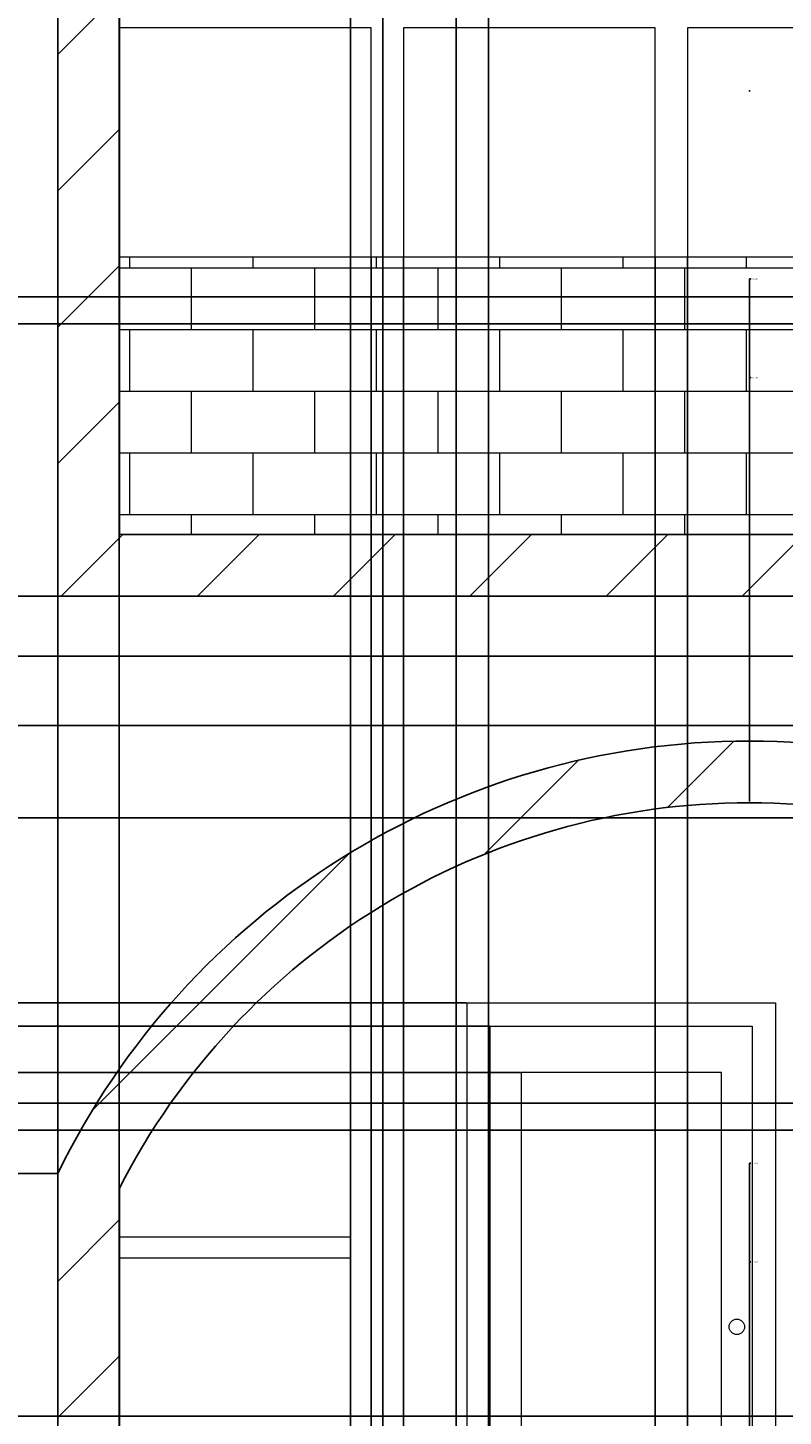
# Model space of a CAD drawing. Units: inches. Extents: x -14 to 375, y -86 to 549.
# Tile 7 of 12: x 130 to 228, y 156 to 336. Entities that reach past the tile are written whole.
import ezdxf

# ---------------------------------------------------------------- set-up
doc = ezdxf.new("R2010")
doc.units = ezdxf.units.IN
doc.header["$MEASUREMENT"] = 0
for name, color, linetype, lineweight in [('A-ANNO-DIMS', 2, 'Continuous', 18), ('A-DOOR', 3, 'Continuous', 18), ('A-ELEV', 7, 'Continuous', 25), ('A-ELEV-PATT', 8, 'Continuous', 13), ('A-ELEV-RAIL', 8, 'Continuous', 18), ('A-GLAZ', 4, 'Continuous', 18)]:
    doc.layers.add(name, color=color, linetype=linetype, lineweight=lineweight)
doc.styles.get("Standard").update_dxf_attribs({"font": 'arial.ttf'})
doc.dimstyles.get("Standard").update_dxf_attribs({"dimtxt": 0.18, "dimasz": 0.18, "dimexe": 0.18, "dimexo": 0.0625, "dimgap": 0.09, "dimtad": 0, "dimtih": 1, "dimtoh": 1, "dimdec": 4, "dimzin": 0, "dimdsep": 46, "dimtxsty": 'Standard', "dimcen": 0.09, "dimadec": 0, "dimazin": 0, "dimtfac": 1, "dimtdec": 4, "dimtofl": 0, "dimtmove": 0, "dimatfit": 3, "dimfxl": 1, "dimtolj": 1, "dimtzin": 0, "dimarcsym": 0})

# ---------------------------------------------------------------- blocks, each defined once
blk = doc.blocks.new('*U3')
blk.add_lwpolyline([(3.12, 0.01), (0.12, 0.01), (0.12, 84.01), (40.12, 84.01), (40.12, 0.01), (37.12, 0.01)])
for points in [[(37.12, 80.99), (37.12, 0.01), (3.12, 0.01), (3.12, 80.99)], [(33.12, 6.01), (33.12, 74.99), (7.12, 74.99), (7.12, 6.01)]]:
    blk.add_lwpolyline(points, close=True)
blk.add_circle((35.12, 42.01), 1)
blk = doc.blocks.new('*D15')
at = {"layer": 'A-ANNO-DIMS', "color": 0, "lineweight": -2, "transparency": 16777216}
for p, q in [((134.17, 187.85), (-13.88, 187.85)), ((-13.7, 187.67), (-13.7, 170.29)), ((-13.7, 152.56), (-13.7, 169.93)), ((38.44, 152.38), (-13.88, 152.38))]:
    blk.add_line(p, q, dxfattribs=at)
at = {"layer": 'A-ANNO-DIMS', "color": 0, "transparency": 16777216}
for points in [[(-13.73, 187.67), (-13.67, 187.67), (-13.7, 187.85)], [(-13.73, 152.56), (-13.67, 152.56), (-13.7, 152.38)]]:
    blk.add_solid(points, dxfattribs=at)
at = {"layer": 'Defpoints', "color": 0, "transparency": 16777216}
for p in [(-13.7, 187.85), (134.23, 187.85), (38.5, 152.38)]:
    blk.add_point(p, dxfattribs=at)
at = {"layer": 'A-ANNO-DIMS', "color": 0, "transparency": 16777216, "insert": (-13.7, 170.11), "char_height": 0.18, "attachment_point": 5}
blk.add_mtext('\\A1;35.47', dxfattribs=at)
blk = doc.blocks.new('*D16')
at = {"layer": 'A-ANNO-DIMS', "color": 0, "lineweight": -2, "transparency": 16777216}
for p, q in [((134.17, 262.71), (-13.88, 262.71)), ((-13.7, 262.53), (-13.7, 225.46)), ((-13.7, 188.03), (-13.7, 225.09)), ((134.17, 187.85), (-13.88, 187.85))]:
    blk.add_line(p, q, dxfattribs=at)
at = {"layer": 'A-ANNO-DIMS', "color": 0, "transparency": 16777216}
for points in [[(-13.73, 262.53), (-13.67, 262.53), (-13.7, 262.71)], [(-13.73, 188.03), (-13.67, 188.03), (-13.7, 187.85)]]:
    blk.add_solid(points, dxfattribs=at)
at = {"layer": 'Defpoints', "color": 0, "transparency": 16777216}
for p in [(-13.7, 262.71), (134.23, 262.71), (134.23, 187.85)]:
    blk.add_point(p, dxfattribs=at)
at = {"layer": 'A-ANNO-DIMS', "color": 0, "transparency": 16777216, "insert": (-13.7, 225.28), "char_height": 0.18, "attachment_point": 5}
blk.add_mtext('\\A1;74.86', dxfattribs=at)
blk = doc.blocks.new('*D17')
at = {"layer": 'A-ANNO-DIMS', "color": 0, "lineweight": -2, "transparency": 16777216}
for p, q in [((38.44, 432.97), (-13.88, 432.97)), ((-13.7, 432.79), (-13.7, 348.02)), ((-13.7, 262.89), (-13.7, 347.66)), ((134.17, 262.71), (-13.88, 262.71))]:
    blk.add_line(p, q, dxfattribs=at)
at = {"layer": 'A-ANNO-DIMS', "color": 0, "transparency": 16777216}
for points in [[(-13.73, 432.79), (-13.67, 432.79), (-13.7, 432.97)], [(-13.73, 262.89), (-13.67, 262.89), (-13.7, 262.71)]]:
    blk.add_solid(points, dxfattribs=at)
at = {"layer": 'Defpoints', "color": 0, "transparency": 16777216}
for p in [(-13.7, 432.97), (38.5, 432.97), (134.23, 262.71)]:
    blk.add_point(p, dxfattribs=at)
at = {"layer": 'A-ANNO-DIMS', "color": 0, "transparency": 16777216, "insert": (-13.7, 347.84), "char_height": 0.18, "attachment_point": 5}
blk.add_mtext('\\A1;170.26', dxfattribs=at)
blk = doc.blocks.new('*D29')
at = {"layer": 'A-ANNO-DIMS', "color": 0, "lineweight": -2, "transparency": 16777216}
for p, q in [((107.74, 193.48), (374.54, 193.48)), ((374.36, 193.3), (374.36, 175.11)), ((374.36, 156.56), (374.36, 174.75)), ((107.76, 156.38), (374.54, 156.38))]:
    blk.add_line(p, q, dxfattribs=at)
at = {"layer": 'A-ANNO-DIMS', "color": 0, "transparency": 16777216}
for points in [[(374.33, 193.3), (374.39, 193.3), (374.36, 193.48)], [(374.33, 156.56), (374.39, 156.56), (374.36, 156.38)]]:
    blk.add_solid(points, dxfattribs=at)
at = {"layer": 'Defpoints', "color": 0, "transparency": 16777216}
for p in [(107.68, 193.48), (374.36, 193.48), (107.7, 156.38)]:
    blk.add_point(p, dxfattribs=at)
at = {"layer": 'A-ANNO-DIMS', "color": 0, "transparency": 16777216, "insert": (374.36, 174.93), "char_height": 0.18, "attachment_point": 5}
blk.add_mtext('\\A1;37.106', dxfattribs=at)
blk = doc.blocks.new('*D30')
at = {"layer": 'A-ANNO-DIMS', "color": 0, "lineweight": -2, "transparency": 16777216}
for p, q in [((107.74, 196.98), (374.54, 196.98)), ((374.36, 196.8), (374.36, 195.41)), ((374.36, 193.66), (374.36, 195.05)), ((107.74, 193.48), (374.54, 193.48))]:
    blk.add_line(p, q, dxfattribs=at)
at = {"layer": 'A-ANNO-DIMS', "color": 0, "transparency": 16777216}
for points in [[(374.33, 196.8), (374.39, 196.8), (374.36, 196.98)], [(374.33, 193.66), (374.39, 193.66), (374.36, 193.48)]]:
    blk.add_solid(points, dxfattribs=at)
at = {"layer": 'Defpoints', "color": 0, "transparency": 16777216}
for p in [(107.68, 196.98), (374.36, 196.98), (107.68, 193.48)]:
    blk.add_point(p, dxfattribs=at)
at = {"layer": 'A-ANNO-DIMS', "color": 0, "transparency": 16777216, "insert": (374.36, 195.23), "char_height": 0.18, "attachment_point": 5}
blk.add_mtext('\\A1;3.501', dxfattribs=at)
blk = doc.blocks.new('*D31')
at = {"layer": 'A-ANNO-DIMS', "color": 0, "lineweight": -2, "transparency": 16777216}
for p, q in [((107.76, 233.96), (374.54, 233.96)), ((374.36, 233.78), (374.36, 215.65)), ((374.36, 197.16), (374.36, 215.29)), ((107.74, 196.98), (374.54, 196.98))]:
    blk.add_line(p, q, dxfattribs=at)
at = {"layer": 'A-ANNO-DIMS', "color": 0, "transparency": 16777216}
for points in [[(374.33, 233.78), (374.39, 233.78), (374.36, 233.96)], [(374.33, 197.16), (374.39, 197.16), (374.36, 196.98)]]:
    blk.add_solid(points, dxfattribs=at)
at = {"layer": 'Defpoints', "color": 0, "transparency": 16777216}
for p in [(107.7, 233.96), (374.36, 233.96), (107.68, 196.98)]:
    blk.add_point(p, dxfattribs=at)
at = {"layer": 'A-ANNO-DIMS', "color": 0, "transparency": 16777216, "insert": (374.36, 215.47), "char_height": 0.18, "attachment_point": 5}
blk.add_mtext('\\A1;36.975', dxfattribs=at)
blk = doc.blocks.new('*D32')
at = {"layer": 'A-ANNO-DIMS', "color": 0, "lineweight": -2, "transparency": 16777216}
for p, q in [((107.76, 245.96), (374.54, 245.96)), ((374.36, 245.78), (374.36, 240.14)), ((374.36, 234.14), (374.36, 239.78)), ((107.76, 233.96), (374.54, 233.96))]:
    blk.add_line(p, q, dxfattribs=at)
at = {"layer": 'A-ANNO-DIMS', "color": 0, "transparency": 16777216}
for points in [[(374.33, 245.78), (374.39, 245.78), (374.36, 245.96)], [(374.33, 234.14), (374.39, 234.14), (374.36, 233.96)]]:
    blk.add_solid(points, dxfattribs=at)
at = {"layer": 'Defpoints', "color": 0, "transparency": 16777216}
for p in [(107.7, 245.96), (374.36, 245.96), (107.7, 233.96)]:
    blk.add_point(p, dxfattribs=at)
at = {"layer": 'A-ANNO-DIMS', "color": 0, "transparency": 16777216, "insert": (374.36, 239.96), "char_height": 0.18, "attachment_point": 5}
blk.add_mtext('\\A1;12', dxfattribs=at)
blk = doc.blocks.new('*D33')
at = {"layer": 'A-ANNO-DIMS', "color": 0, "lineweight": -2, "transparency": 16777216}
for p, q in [((107.76, 254.96), (374.54, 254.96)), ((374.36, 254.78), (374.36, 250.64)), ((374.36, 246.14), (374.36, 250.28)), ((107.76, 245.96), (374.54, 245.96))]:
    blk.add_line(p, q, dxfattribs=at)
at = {"layer": 'A-ANNO-DIMS', "color": 0, "transparency": 16777216}
for points in [[(374.33, 254.78), (374.39, 254.78), (374.36, 254.96)], [(374.33, 246.14), (374.39, 246.14), (374.36, 245.96)]]:
    blk.add_solid(points, dxfattribs=at)
at = {"layer": 'Defpoints', "color": 0, "transparency": 16777216}
for p in [(107.7, 254.96), (374.36, 254.96), (107.7, 245.96)]:
    blk.add_point(p, dxfattribs=at)
at = {"layer": 'A-ANNO-DIMS', "color": 0, "transparency": 16777216, "insert": (374.36, 250.46), "char_height": 0.18, "attachment_point": 5}
blk.add_mtext('\\A1;9', dxfattribs=at)
blk = doc.blocks.new('*D34')
at = {"layer": 'A-ANNO-DIMS', "color": 0, "lineweight": -2, "transparency": 16777216}
for p, q in [((107.64, 298.04), (374.54, 298.04)), ((374.36, 297.86), (374.36, 276.68)), ((374.36, 255.14), (374.36, 276.32)), ((107.76, 254.96), (374.54, 254.96))]:
    blk.add_line(p, q, dxfattribs=at)
at = {"layer": 'A-ANNO-DIMS', "color": 0, "transparency": 16777216}
for points in [[(374.33, 297.86), (374.39, 297.86), (374.36, 298.04)], [(374.33, 255.14), (374.39, 255.14), (374.36, 254.96)]]:
    blk.add_solid(points, dxfattribs=at)
at = {"layer": 'Defpoints', "color": 0, "transparency": 16777216}
for p in [(107.58, 298.04), (374.36, 298.04), (107.7, 254.96)]:
    blk.add_point(p, dxfattribs=at)
at = {"layer": 'A-ANNO-DIMS', "color": 0, "transparency": 16777216, "insert": (374.36, 276.5), "char_height": 0.18, "attachment_point": 5}
blk.add_mtext('\\A1;43.08', dxfattribs=at)
blk = doc.blocks.new('*D35')
at = {"layer": 'A-ANNO-DIMS', "color": 0, "lineweight": -2, "transparency": 16777216}
for p, q in [((107.64, 301.54), (374.54, 301.54)), ((374.36, 301.36), (374.36, 299.97)), ((374.36, 298.22), (374.36, 299.6)), ((107.64, 298.04), (374.54, 298.04))]:
    blk.add_line(p, q, dxfattribs=at)
at = {"layer": 'A-ANNO-DIMS', "color": 0, "transparency": 16777216}
for points in [[(374.33, 301.36), (374.39, 301.36), (374.36, 301.54)], [(374.33, 298.22), (374.39, 298.22), (374.36, 298.04)]]:
    blk.add_solid(points, dxfattribs=at)
at = {"layer": 'Defpoints', "color": 0, "transparency": 16777216}
for p in [(107.58, 301.54), (374.36, 301.54), (107.58, 298.04)]:
    blk.add_point(p, dxfattribs=at)
at = {"layer": 'A-ANNO-DIMS', "color": 0, "transparency": 16777216, "insert": (374.36, 299.79), "char_height": 0.18, "attachment_point": 5}
blk.add_mtext('\\A1;3.501', dxfattribs=at)
blk = doc.blocks.new('*D36')
at = {"layer": 'A-ANNO-DIMS', "color": 0, "lineweight": -2, "transparency": 16777216}
for p, q in [((107.56, 353.96), (374.54, 353.96)), ((374.36, 353.78), (374.36, 327.93)), ((374.36, 301.72), (374.36, 327.57)), ((107.64, 301.54), (374.54, 301.54))]:
    blk.add_line(p, q, dxfattribs=at)
at = {"layer": 'A-ANNO-DIMS', "color": 0, "transparency": 16777216}
for points in [[(374.33, 353.78), (374.39, 353.78), (374.36, 353.96)], [(374.33, 301.72), (374.39, 301.72), (374.36, 301.54)]]:
    blk.add_solid(points, dxfattribs=at)
at = {"layer": 'Defpoints', "color": 0, "transparency": 16777216}
for p in [(107.5, 353.96), (374.36, 353.96), (107.58, 301.54)]:
    blk.add_point(p, dxfattribs=at)
at = {"layer": 'A-ANNO-DIMS', "color": 0, "transparency": 16777216, "insert": (374.36, 327.75), "char_height": 0.18, "attachment_point": 5}
blk.add_mtext('\\A1;52.42', dxfattribs=at)
blk = doc.blocks.new('*D42')
at = {"layer": 'A-ANNO-DIMS', "color": 0, "lineweight": -2, "transparency": 16777216}
for p, q in [((142.23, 270.64), (142.23, -64.39)), ((134.23, 262.64), (134.23, -64.39)), ((134.41, -64.21), (138.08, -64.21)), ((142.05, -64.21), (138.38, -64.21))]:
    blk.add_line(p, q, dxfattribs=at)
at = {"layer": 'A-ANNO-DIMS', "color": 0, "transparency": 16777216}
for points in [[(134.41, -64.18), (134.41, -64.24), (134.23, -64.21)], [(142.05, -64.18), (142.05, -64.24), (142.23, -64.21)]]:
    blk.add_solid(points, dxfattribs=at)
at = {"layer": 'Defpoints', "color": 0, "transparency": 16777216}
for p in [(142.23, 270.71), (134.23, 262.71), (142.23, -64.21)]:
    blk.add_point(p, dxfattribs=at)
at = {"layer": 'A-ANNO-DIMS', "color": 0, "transparency": 16777216, "insert": (138.23, -64.21), "char_height": 0.18, "attachment_point": 5}
blk.add_mtext('\\A1;8', dxfattribs=at)
blk = doc.blocks.new('*D43')
at = {"layer": 'A-ANNO-DIMS', "color": 0, "lineweight": -2, "transparency": 16777216}
for p, q in [((142.23, 270.64), (142.23, -64.39)), ((305.63, 270.64), (305.63, -64.39)), ((142.41, -64.21), (223.55, -64.21)), ((305.45, -64.21), (224.32, -64.21))]:
    blk.add_line(p, q, dxfattribs=at)
at = {"layer": 'A-ANNO-DIMS', "color": 0, "transparency": 16777216}
for points in [[(142.41, -64.18), (142.41, -64.24), (142.23, -64.21)], [(305.45, -64.18), (305.45, -64.24), (305.63, -64.21)]]:
    blk.add_solid(points, dxfattribs=at)
at = {"layer": 'Defpoints', "color": 0, "transparency": 16777216}
for p in [(142.23, 270.71), (305.63, 270.71), (305.63, -64.21)]:
    blk.add_point(p, dxfattribs=at)
at = {"layer": 'A-ANNO-DIMS', "color": 0, "transparency": 16777216, "insert": (223.93, -64.21), "char_height": 0.18, "attachment_point": 5}
blk.add_mtext('\\A1;163.4', dxfattribs=at)
blk = doc.blocks.new('*D45')
at = {"layer": 'A-ANNO-DIMS', "color": 0, "lineweight": -2, "transparency": 16777216}
for p, q in [((142.23, 306.64), (142.23, -64.39)), ((174.92, 306.64), (174.92, -64.39)), ((142.41, -64.21), (158.19, -64.21)), ((174.74, -64.21), (158.97, -64.21))]:
    blk.add_line(p, q, dxfattribs=at)
at = {"layer": 'A-ANNO-DIMS', "color": 0, "transparency": 16777216}
for points in [[(142.41, -64.18), (142.41, -64.24), (142.23, -64.21)], [(174.74, -64.18), (174.74, -64.24), (174.92, -64.21)]]:
    blk.add_solid(points, dxfattribs=at)
at = {"layer": 'Defpoints', "color": 0, "transparency": 16777216}
for p in [(142.23, 306.71), (174.92, 306.71), (174.92, -64.21)]:
    blk.add_point(p, dxfattribs=at)
at = {"layer": 'A-ANNO-DIMS', "color": 0, "transparency": 16777216, "insert": (158.58, -64.21), "char_height": 0.18, "attachment_point": 5}
blk.add_mtext('\\A1;32.69', dxfattribs=at)
blk = doc.blocks.new('*D46')
at = {"layer": 'A-ANNO-DIMS', "color": 0, "lineweight": -2, "transparency": 16777216}
for p, q in [((174.92, 306.64), (174.92, -64.39)), ((179.09, 306.64), (179.09, -64.39)), ((175.1, -64.21), (176.68, -64.21)), ((178.91, -64.21), (177.33, -64.21))]:
    blk.add_line(p, q, dxfattribs=at)
at = {"layer": 'A-ANNO-DIMS', "color": 0, "transparency": 16777216}
for points in [[(175.1, -64.18), (175.1, -64.24), (174.92, -64.21)], [(178.91, -64.18), (178.91, -64.24), (179.09, -64.21)]]:
    blk.add_solid(points, dxfattribs=at)
at = {"layer": 'Defpoints', "color": 0, "transparency": 16777216}
for p in [(174.92, 306.71), (179.09, 306.71), (179.09, -64.21)]:
    blk.add_point(p, dxfattribs=at)
at = {"layer": 'A-ANNO-DIMS', "color": 0, "transparency": 16777216, "insert": (177.01, -64.21), "char_height": 0.18, "attachment_point": 5}
blk.add_mtext('\\A1;4.17', dxfattribs=at)
blk = doc.blocks.new('*D47')
at = {"layer": 'A-ANNO-DIMS', "color": 0, "lineweight": -2, "transparency": 16777216}
for p, q in [((179.09, 306.64), (179.09, -64.39)), ((211.78, 306.64), (211.78, -64.39)), ((179.27, -64.21), (195.04, -64.21)), ((211.6, -64.21), (195.83, -64.21))]:
    blk.add_line(p, q, dxfattribs=at)
at = {"layer": 'A-ANNO-DIMS', "color": 0, "transparency": 16777216}
for points in [[(179.27, -64.18), (179.27, -64.24), (179.09, -64.21)], [(211.6, -64.18), (211.6, -64.24), (211.78, -64.21)]]:
    blk.add_solid(points, dxfattribs=at)
at = {"layer": 'Defpoints', "color": 0, "transparency": 16777216}
for p in [(179.09, 306.71), (211.78, 306.71), (211.78, -64.21)]:
    blk.add_point(p, dxfattribs=at)
at = {"layer": 'A-ANNO-DIMS', "color": 0, "transparency": 16777216, "insert": (195.44, -64.21), "char_height": 0.18, "attachment_point": 5}
blk.add_mtext('\\A1;32.69', dxfattribs=at)
blk = doc.blocks.new('*D48')
at = {"layer": 'A-ANNO-DIMS', "color": 0, "lineweight": -2, "transparency": 16777216}
for p, q in [((211.78, 306.64), (211.78, -64.39)), ((215.95, 306.64), (215.95, -64.39)), ((211.96, -64.21), (213.54, -64.21)), ((215.77, -64.21), (214.19, -64.21))]:
    blk.add_line(p, q, dxfattribs=at)
at = {"layer": 'A-ANNO-DIMS', "color": 0, "transparency": 16777216}
for points in [[(211.96, -64.18), (211.96, -64.24), (211.78, -64.21)], [(215.77, -64.18), (215.77, -64.24), (215.95, -64.21)]]:
    blk.add_solid(points, dxfattribs=at)
at = {"layer": 'Defpoints', "color": 0, "transparency": 16777216}
for p in [(211.78, 306.71), (215.95, 306.71), (215.95, -64.21)]:
    blk.add_point(p, dxfattribs=at)
at = {"layer": 'A-ANNO-DIMS', "color": 0, "transparency": 16777216, "insert": (213.86, -64.21), "char_height": 0.18, "attachment_point": 5}
blk.add_mtext('\\A1;4.17', dxfattribs=at)
blk = doc.blocks.new('*D49')
at = {"layer": 'A-ANNO-DIMS', "color": 0, "lineweight": -2, "transparency": 16777216}
for p, q in [((215.95, 306.64), (215.95, -64.39)), ((248.64, 306.64), (248.64, -64.39)), ((216.13, -64.21), (231.9, -64.21)), ((248.46, -64.21), (232.69, -64.21))]:
    blk.add_line(p, q, dxfattribs=at)
at = {"layer": 'A-ANNO-DIMS', "color": 0, "transparency": 16777216}
for points in [[(216.13, -64.18), (216.13, -64.24), (215.95, -64.21)], [(248.46, -64.18), (248.46, -64.24), (248.64, -64.21)]]:
    blk.add_solid(points, dxfattribs=at)
at = {"layer": 'Defpoints', "color": 0, "transparency": 16777216}
for p in [(215.95, 306.71), (248.64, 306.71), (248.64, -64.21)]:
    blk.add_point(p, dxfattribs=at)
at = {"layer": 'A-ANNO-DIMS', "color": 0, "transparency": 16777216, "insert": (232.29, -64.21), "char_height": 0.18, "attachment_point": 5}
blk.add_mtext('\\A1;32.69', dxfattribs=at)
blk = doc.blocks.new('*D96')
at = {"layer": 'A-ANNO-DIMS', "color": 0, "lineweight": -2, "transparency": 16777216}
for p, q in [((194.3, 200.95), (-13.88, 200.95)), ((-13.7, 200.77), (-13.7, 166.64)), ((-13.7, 132.15), (-13.7, 166.28)), ((194.3, 131.97), (-13.88, 131.97))]:
    blk.add_line(p, q, dxfattribs=at)
at = {"layer": 'A-ANNO-DIMS', "color": 0, "transparency": 16777216}
for points in [[(-13.73, 200.77), (-13.67, 200.77), (-13.7, 200.95)], [(-13.73, 132.15), (-13.67, 132.15), (-13.7, 131.97)]]:
    blk.add_solid(points, dxfattribs=at)
at = {"layer": 'Defpoints', "color": 0, "transparency": 16777216}
for p in [(-13.7, 200.95), (194.37, 200.95), (194.37, 131.97)]:
    blk.add_point(p, dxfattribs=at)
at = {"layer": 'A-ANNO-DIMS', "color": 0, "transparency": 16777216, "insert": (-13.7, 166.46), "char_height": 0.18, "attachment_point": 5}
blk.add_mtext('\\A1;68.98', dxfattribs=at)
blk = doc.blocks.new('*D97')
at = {"layer": 'A-ANNO-DIMS', "color": 0, "lineweight": -2, "transparency": 16777216}
for p, q in [((190.3, 206.95), (-13.88, 206.95)), ((-13.7, 206.77), (-13.7, 204.13)), ((-13.7, 201.13), (-13.7, 203.77)), ((194.3, 200.95), (-13.88, 200.95))]:
    blk.add_line(p, q, dxfattribs=at)
at = {"layer": 'A-ANNO-DIMS', "color": 0, "transparency": 16777216}
for points in [[(-13.73, 206.77), (-13.67, 206.77), (-13.7, 206.95)], [(-13.73, 201.13), (-13.67, 201.13), (-13.7, 200.95)]]:
    blk.add_solid(points, dxfattribs=at)
at = {"layer": 'Defpoints', "color": 0, "transparency": 16777216}
for p in [(-13.7, 206.95), (190.37, 206.95), (194.37, 200.95)]:
    blk.add_point(p, dxfattribs=at)
at = {"layer": 'A-ANNO-DIMS', "color": 0, "transparency": 16777216, "insert": (-13.7, 203.95), "char_height": 0.18, "attachment_point": 5}
blk.add_mtext('\\A1;6', dxfattribs=at)
blk = doc.blocks.new('*D98')
at = {"layer": 'A-ANNO-DIMS', "color": 0, "lineweight": -2, "transparency": 16777216}
for p, q in [((187.3, 209.97), (-13.88, 209.97)), ((-13.7, 209.79), (-13.7, 208.64)), ((-13.7, 207.13), (-13.7, 208.28)), ((190.3, 206.95), (-13.88, 206.95))]:
    blk.add_line(p, q, dxfattribs=at)
at = {"layer": 'A-ANNO-DIMS', "color": 0, "transparency": 16777216}
for points in [[(-13.73, 209.79), (-13.67, 209.79), (-13.7, 209.97)], [(-13.73, 207.13), (-13.67, 207.13), (-13.7, 206.95)]]:
    blk.add_solid(points, dxfattribs=at)
at = {"layer": 'Defpoints', "color": 0, "transparency": 16777216}
for p in [(-13.7, 209.97), (187.37, 209.97), (190.37, 206.95)]:
    blk.add_point(p, dxfattribs=at)
at = {"layer": 'A-ANNO-DIMS', "color": 0, "transparency": 16777216, "insert": (-13.7, 208.46), "char_height": 0.18, "attachment_point": 5}
blk.add_mtext('\\A1;3.023', dxfattribs=at)
blk = doc.blocks.new('*D99')
at = {"layer": 'A-ANNO-DIMS', "color": 0, "lineweight": -2, "transparency": 16777216}
for p, q in [((134.23, 6.02), (134.23, 515.24)), ((134.41, 515.06), (138.08, 515.06)), ((142.05, 515.06), (138.38, 515.06)), ((142.23, 6.02), (142.23, 515.24))]:
    blk.add_line(p, q, dxfattribs=at)
at = {"layer": 'A-ANNO-DIMS', "color": 0, "transparency": 16777216}
for points in [[(134.41, 515.09), (134.41, 515.03), (134.23, 515.06)], [(142.05, 515.09), (142.05, 515.03), (142.23, 515.06)]]:
    blk.add_solid(points, dxfattribs=at)
at = {"layer": 'Defpoints', "color": 0, "transparency": 16777216}
for p in [(142.23, 515.06), (134.23, 5.96), (142.23, 5.96)]:
    blk.add_point(p, dxfattribs=at)
at = {"layer": 'A-ANNO-DIMS', "color": 0, "transparency": 16777216, "insert": (138.23, 515.06), "char_height": 0.18, "attachment_point": 5}
blk.add_mtext('\\A1;8', dxfattribs=at)
blk = doc.blocks.new('*D100')
at = {"layer": 'A-ANNO-DIMS', "color": 0, "lineweight": -2, "transparency": 16777216}
for p, q in [((142.23, 6.02), (142.23, 515.24)), ((142.41, 515.06), (157.01, 515.06)), ((172.05, 515.06), (157.45, 515.06)), ((172.23, 6.02), (172.23, 515.24))]:
    blk.add_line(p, q, dxfattribs=at)
at = {"layer": 'A-ANNO-DIMS', "color": 0, "transparency": 16777216}
for points in [[(142.41, 515.09), (142.41, 515.03), (142.23, 515.06)], [(172.05, 515.09), (172.05, 515.03), (172.23, 515.06)]]:
    blk.add_solid(points, dxfattribs=at)
at = {"layer": 'Defpoints', "color": 0, "transparency": 16777216}
for p in [(172.23, 515.06), (142.23, 5.96), (172.23, 5.96)]:
    blk.add_point(p, dxfattribs=at)
at = {"layer": 'A-ANNO-DIMS', "color": 0, "transparency": 16777216, "insert": (157.23, 515.06), "char_height": 0.18, "attachment_point": 5}
blk.add_mtext('\\A1;30', dxfattribs=at)
blk = doc.blocks.new('*D101')
at = {"layer": 'A-ANNO-DIMS', "color": 0, "lineweight": -2, "transparency": 16777216}
for p, q in [((172.23, 6.02), (172.23, 515.24)), ((172.41, 515.06), (173.93, 515.06)), ((176.24, 515.06), (174.72, 515.06)), ((176.42, 6.02), (176.42, 515.24))]:
    blk.add_line(p, q, dxfattribs=at)
at = {"layer": 'A-ANNO-DIMS', "color": 0, "transparency": 16777216}
for points in [[(172.41, 515.09), (172.41, 515.03), (172.23, 515.06)], [(176.24, 515.09), (176.24, 515.03), (176.42, 515.06)]]:
    blk.add_solid(points, dxfattribs=at)
at = {"layer": 'Defpoints', "color": 0, "transparency": 16777216}
for p in [(176.42, 515.06), (172.23, 5.96), (176.42, 5.96)]:
    blk.add_point(p, dxfattribs=at)
at = {"layer": 'A-ANNO-DIMS', "color": 0, "transparency": 16777216, "insert": (174.32, 515.06), "char_height": 0.18, "attachment_point": 5}
blk.add_mtext('\\A1;4.186', dxfattribs=at)
blk = doc.blocks.new('*D102')
at = {"layer": 'A-ANNO-DIMS', "color": 0, "lineweight": -2, "transparency": 16777216}
for p, q in [((176.42, 6.02), (176.42, 515.24)), ((176.6, 515.06), (180.8, 515.06)), ((185.78, 515.06), (181.58, 515.06)), ((185.96, 6.02), (185.96, 515.24))]:
    blk.add_line(p, q, dxfattribs=at)
at = {"layer": 'A-ANNO-DIMS', "color": 0, "transparency": 16777216}
for points in [[(176.6, 515.09), (176.6, 515.03), (176.42, 515.06)], [(185.78, 515.09), (185.78, 515.03), (185.96, 515.06)]]:
    blk.add_solid(points, dxfattribs=at)
at = {"layer": 'Defpoints', "color": 0, "transparency": 16777216}
for p in [(185.96, 515.06), (176.42, 5.96), (185.96, 5.96)]:
    blk.add_point(p, dxfattribs=at)
at = {"layer": 'A-ANNO-DIMS', "color": 0, "transparency": 16777216, "insert": (181.19, 515.06), "char_height": 0.18, "attachment_point": 5}
blk.add_mtext('\\A1;9.545', dxfattribs=at)
blk = doc.blocks.new('*D103')
at = {"layer": 'A-ANNO-DIMS', "color": 0, "lineweight": -2, "transparency": 16777216}
for p, q in [((185.96, 6.02), (185.96, 515.24)), ((186.14, 515.06), (187.66, 515.06)), ((189.97, 515.06), (188.45, 515.06)), ((190.15, 6.02), (190.15, 515.24))]:
    blk.add_line(p, q, dxfattribs=at)
at = {"layer": 'A-ANNO-DIMS', "color": 0, "transparency": 16777216}
for points in [[(186.14, 515.09), (186.14, 515.03), (185.96, 515.06)], [(189.97, 515.09), (189.97, 515.03), (190.15, 515.06)]]:
    blk.add_solid(points, dxfattribs=at)
at = {"layer": 'Defpoints', "color": 0, "transparency": 16777216}
for p in [(190.15, 515.06), (185.96, 5.96), (190.15, 5.96)]:
    blk.add_point(p, dxfattribs=at)
at = {"layer": 'A-ANNO-DIMS', "color": 0, "transparency": 16777216, "insert": (188.06, 515.06), "char_height": 0.18, "attachment_point": 5}
blk.add_mtext('\\A1;4.186', dxfattribs=at)
blk = doc.blocks.new('*D104')
at = {"layer": 'A-ANNO-DIMS', "color": 0, "lineweight": -2, "transparency": 16777216}
for p, q in [((190.15, 6.02), (190.15, 515.24)), ((190.33, 515.06), (230.18, 515.06)), ((270.82, 515.06), (230.97, 515.06)), ((271, 6.02), (271, 515.24))]:
    blk.add_line(p, q, dxfattribs=at)
at = {"layer": 'A-ANNO-DIMS', "color": 0, "transparency": 16777216}
for points in [[(190.33, 515.09), (190.33, 515.03), (190.15, 515.06)], [(270.82, 515.09), (270.82, 515.03), (271, 515.06)]]:
    blk.add_solid(points, dxfattribs=at)
at = {"layer": 'Defpoints', "color": 0, "transparency": 16777216}
for p in [(271, 515.06), (190.15, 5.96), (271, 5.96)]:
    blk.add_point(p, dxfattribs=at)
at = {"layer": 'A-ANNO-DIMS', "color": 0, "transparency": 16777216, "insert": (230.57, 515.06), "char_height": 0.18, "attachment_point": 5}
blk.add_mtext('\\A1;80.85', dxfattribs=at)
blk = doc.blocks.new('*D133')
at = {"layer": 'A-ANNO-DIMS', "color": 0, "lineweight": -2, "transparency": 16777216}
for p, q in [((224.18, 549.18), (224, 549.18)), ((224, 549.18), (224, 466.51)), ((223.91, 328.25), (224.09, 328.25)), ((224, 328.16), (224, 328.34))]:
    blk.add_line(p, q, dxfattribs=at)
at = {"layer": 'A-ANNO-DIMS', "color": 0, "transparency": 16777216}
blk.add_solid([(223.97, 466.51), (224.03, 466.51), (224, 466.33)], dxfattribs=at)
at = {"layer": 'Defpoints', "color": 0, "transparency": 16777216}
for p in [(224, 466.33), (224, 328.25)]:
    blk.add_point(p, dxfattribs=at)
at = {"layer": 'A-ANNO-DIMS', "color": 0, "transparency": 16777216, "insert": (224.73, 549.18), "char_height": 0.18, "attachment_point": 5}
blk.add_mtext('\\A1;R138.08', dxfattribs=at)
blk = doc.blocks.new('*D134')
at = {"layer": 'A-ANNO-DIMS', "color": 0, "lineweight": -2, "transparency": 16777216}
for p, q in [((224.18, 536.38), (224, 536.38)), ((224, 536.38), (224, 458.51)), ((223.91, 328.25), (224.09, 328.25)), ((224, 328.16), (224, 328.34))]:
    blk.add_line(p, q, dxfattribs=at)
at = {"layer": 'A-ANNO-DIMS', "color": 0, "transparency": 16777216}
blk.add_solid([(223.97, 458.51), (224.03, 458.51), (224, 458.33)], dxfattribs=at)
at = {"layer": 'Defpoints', "color": 0, "transparency": 16777216}
for p in [(224, 458.33), (224, 328.25)]:
    blk.add_point(p, dxfattribs=at)
at = {"layer": 'A-ANNO-DIMS', "color": 0, "transparency": 16777216, "insert": (224.73, 536.38), "char_height": 0.18, "attachment_point": 5}
blk.add_mtext('\\A1;R130.08', dxfattribs=at)
blk = doc.blocks.new('*D135')
at = {"layer": 'A-ANNO-DIMS', "color": 0, "lineweight": -2, "transparency": 16777216}
for p, q in [((224.18, 303.87), (224, 303.87)), ((224, 303.87), (224, 244.12)), ((223.91, 144.06), (224.09, 144.06)), ((224, 143.97), (224, 144.15))]:
    blk.add_line(p, q, dxfattribs=at)
at = {"layer": 'A-ANNO-DIMS', "color": 0, "transparency": 16777216}
blk.add_solid([(223.97, 244.12), (224.03, 244.12), (224, 243.94)], dxfattribs=at)
at = {"layer": 'Defpoints', "color": 0, "transparency": 16777216}
for p in [(224, 243.94), (224, 144.06)]:
    blk.add_point(p, dxfattribs=at)
at = {"layer": 'A-ANNO-DIMS', "color": 0, "transparency": 16777216, "insert": (224.66, 303.87), "char_height": 0.18, "attachment_point": 5}
blk.add_mtext('\\A1;R99.88', dxfattribs=at)
blk = doc.blocks.new('*D136')
at = {"layer": 'A-ANNO-DIMS', "color": 0, "lineweight": -2, "transparency": 16777216}
for p, q in [((224.18, 291.07), (224, 291.07)), ((224, 291.07), (224, 236.12)), ((223.91, 144.06), (224.09, 144.06)), ((224, 143.97), (224, 144.15))]:
    blk.add_line(p, q, dxfattribs=at)
at = {"layer": 'A-ANNO-DIMS', "color": 0, "transparency": 16777216}
blk.add_solid([(223.97, 236.12), (224.03, 236.12), (224, 235.94)], dxfattribs=at)
at = {"layer": 'Defpoints', "color": 0, "transparency": 16777216}
for p in [(224, 235.94), (224, 144.06)]:
    blk.add_point(p, dxfattribs=at)
at = {"layer": 'A-ANNO-DIMS', "color": 0, "transparency": 16777216, "insert": (224.66, 291.07), "char_height": 0.18, "attachment_point": 5}
blk.add_mtext('\\A1;R91.88', dxfattribs=at)
blk = doc.blocks.new('*D137')
at = {"layer": 'A-ANNO-DIMS', "color": 0, "lineweight": -2, "transparency": 16777216}
for p, q in [((224.18, 189.18), (224, 189.18)), ((224, 189.18), (224, 106.51)), ((223.91, -31.75), (224.09, -31.75)), ((224, -31.84), (224, -31.66))]:
    blk.add_line(p, q, dxfattribs=at)
at = {"layer": 'A-ANNO-DIMS', "color": 0, "transparency": 16777216}
blk.add_solid([(223.97, 106.51), (224.03, 106.51), (224, 106.33)], dxfattribs=at)
at = {"layer": 'Defpoints', "color": 0, "transparency": 16777216}
for p in [(224, 106.33), (224, -31.75)]:
    blk.add_point(p, dxfattribs=at)
at = {"layer": 'A-ANNO-DIMS', "color": 0, "transparency": 16777216, "insert": (224.73, 189.18), "char_height": 0.18, "attachment_point": 5}
blk.add_mtext('\\A1;R138.08', dxfattribs=at)
blk = doc.blocks.new('*D138')
at = {"layer": 'A-ANNO-DIMS', "color": 0, "lineweight": -2, "transparency": 16777216}
for p, q in [((224.18, 176.38), (224, 176.38)), ((224, 176.38), (224, 98.51)), ((223.91, -31.75), (224.09, -31.75)), ((224, -31.84), (224, -31.66))]:
    blk.add_line(p, q, dxfattribs=at)
at = {"layer": 'A-ANNO-DIMS', "color": 0, "transparency": 16777216}
blk.add_solid([(223.97, 98.51), (224.03, 98.51), (224, 98.33)], dxfattribs=at)
at = {"layer": 'Defpoints', "color": 0, "transparency": 16777216}
for p in [(224, 98.33), (224, -31.75)]:
    blk.add_point(p, dxfattribs=at)
at = {"layer": 'A-ANNO-DIMS', "color": 0, "transparency": 16777216, "insert": (224.73, 176.38), "char_height": 0.18, "attachment_point": 5}
blk.add_mtext('\\A1;R130.08', dxfattribs=at)

msp = doc.modelspace()

# ---------------------------------------------------------------- hatches: boundary and pattern name
at = {"layer": 'A-ELEV-PATT'}
h = msp.add_hatch(dxfattribs=at)
h.set_pattern_fill('ANSI31', color=256, scale=100)
h.set_pattern_definition([(45, (-168.406, -22.703), (-8.83883, 8.83883), [])])
h.paths.add_polyline_path([(313.6281, 262.7071), (313.6281, 357.9589), (313.7701, 357.9589), (313.7701, 433.1717, 0.36940998), (134.2334, 433.1717), (134.2334, 365.9589), (134.2334, 262.7071)])
h.paths.add_polyline_path([(142.2334, 270.7071), (142.2334, 365.9589), (142.2334, 429.4208, -0.35358711), (305.7701, 429.4208), (305.7701, 365.9589), (305.6281, 365.9589), (305.6281, 270.7071)], flags=16)
h.paths.add_polyline_path([(134.2334, 187.8466), (134.2334, 117.9589), (313.7701, 117.9589), (313.7701, 187.8466, 0.62486768)])
h.paths.add_polyline_path([(305.7701, 185.9589), (305.7701, 125.9589), (142.2334, 125.9589), (142.2334, 185.9589, -0.61125102)], flags=16)
h.paths.add_polyline_path([(134.2334, 73.1717), (134.2334, 5.9589), (142.2334, 5.9589), (142.2334, 69.4208, -0.35358711), (305.7701, 69.4208), (305.7701, 5.9589), (313.7701, 5.9589), (313.7701, 73.1717, 0.36940998)])
h = msp.add_hatch(dxfattribs=at)
h.set_pattern_fill('AR-B816', color=256)
h.set_pattern_definition([(0, (-168.406, -22.703), (0, 8), []), (90, (-168.406, -22.703), (-8, 8), [8, -8])])
h.paths.add_polyline_path([(305.6281, 306.7071), (142.2334, 306.7071), (142.2334, 270.7071), (305.6281, 270.7071)])

# ---------------------------------------------------------------- linework, layer by layer
at = {"layer": 'A-ELEV'}
for points in [[(134.2334, 262.7071), (313.6281, 262.7071), (313.6281, 357.9589), (313.7701, 357.9589), (313.7701, 433.1717, 0.36940998), (134.2334, 433.1717), (134.2334, 365.9589)], [(142.2334, 270.7071), (305.6281, 270.7071), (305.6281, 365.9589), (305.7701, 365.9589), (305.7701, 429.4208, 0.35358711), (142.2334, 429.4208), (142.2334, 365.9589)], [(134.2334, 187.8466), (134.2334, 117.9589), (313.7701, 117.9589), (313.7701, 187.8466, 0.62486768)], [(142.2334, 185.9589), (142.2334, 125.9589), (305.7701, 125.9589), (305.7701, 185.9589, 0.61125102)]]:
    msp.add_lwpolyline(points, format="xyb", close=True, dxfattribs=at)
at = {"layer": 'A-ELEV-RAIL'}
for p, q in [((174.9243, 336.4421), (142.2334, 336.4421)), ((211.7816, 336.4421), (179.0907, 336.4421)), ((248.639, 336.4421), (215.9481, 336.4421)), ((305.6281, 306.7071), (142.2334, 306.7071))]:
    msp.add_line(p, q, dxfattribs=at)
for points in [[(179.0907, 336.4421), (179.0907, 306.7071), (174.9243, 306.7071), (174.9243, 336.4421)], [(215.9481, 336.4421), (215.9481, 306.7071), (211.7816, 306.7071), (211.7816, 336.4421)]]:
    msp.add_lwpolyline(points, dxfattribs=at)
at = {"layer": 'A-GLAZ'}
for points in [[(176.4171, 222.6573), (176.4171, 125.9589)], [(172.2314, 179.5807), (172.2314, 219.9655)], [(172.2314, 179.5807), (142.2334, 179.5807), (142.2334, 176.9318), (172.2314, 176.9318)], [(176.4171, 176.9318), (176.4171, 125.9589), (172.2314, 125.9589), (172.2314, 176.9318)]]:
    msp.add_lwpolyline(points, dxfattribs=at)

# ---------------------------------------------------------------- block references
at = {"layer": 'A-DOOR'}
msp.add_blockref('*U3', (187.242, 125.9589), dxfattribs=at)

# ---------------------------------------------------------------- dimensions: what is measured, and where the dimension line sits
at = {"layer": 'A-ANNO-DIMS'}
for center, mpoint, picture, middle in [((224.0017, 328.25), (224.002, 466.333), '*D133', (224.7321, 549.1828)), ((224.0017, 328.25), (224.002, 458.333), '*D134', (224.7321, 536.3828)), ((224.0017, 144.0634), (224.002, 243.9399), '*D135', (224.6622, 303.8658)), ((224.0017, 144.0634), (224.002, 235.9399), '*D136', (224.6622, 291.0658)), ((224.0017, -31.75), (224.002, 106.333), '*D137', (224.7321, 189.1828)), ((224.0017, -31.75), (224.002, 98.333), '*D138', (224.7321, 176.3828))]:
    dim = msp.add_radius_dim(center=center, mpoint=mpoint, dimstyle='Standard', override={"dimdec": 2, "dimlfac": 1, "dimrnd": 0, "dimzin": 0, "dimdsep": 46, "dimlunit": 2}, dxfattribs=at)
    dim.commit()
    dim.dimension.update_dxf_attribs({"geometry": picture, "text_midpoint": middle, "dimtype": 164})
for base, p1, p2, override, picture, middle in [((142.2334, 515.0589), (134.2334, 5.9589), (142.2334, 5.9589), {"dimdec": 0, "dimlfac": 1, "dimrnd": 0, "dimzin": 0, "dimdsep": 46, "dimlunit": 2}, '*D99', (138.2334, 515.0589)), ((172.2314, 515.0589), (142.2334, 5.9589), (172.2314, 5.9589), {"dimdec": 0, "dimlfac": 1, "dimrnd": 0, "dimzin": 0, "dimdsep": 46, "dimlunit": 2}, '*D100', (157.2324, 515.0589)), ((176.4171, 515.0589), (172.2314, 5.9589), (176.4171, 5.9589), {"dimdec": 3, "dimlfac": 1, "dimrnd": 0, "dimzin": 0, "dimdsep": 46, "dimlunit": 2}, '*D101', (174.3243, 515.0589)), ((185.9623, 515.0589), (176.4171, 5.9589), (185.9623, 5.9589), {"dimdec": 3, "dimlfac": 1, "dimrnd": 0, "dimzin": 0, "dimdsep": 46, "dimlunit": 2}, '*D102', (181.1897, 515.0589)), ((190.148, 515.0589), (185.9623, 5.9589), (190.148, 5.9589), {"dimdec": 3, "dimlfac": 1, "dimrnd": 0, "dimzin": 0, "dimdsep": 46, "dimlunit": 2}, '*D103', (188.0551, 515.0589)), ((270.9993, 515.0589), (190.148, 5.9589), (270.9993, 5.9589), {"dimdec": 2, "dimlfac": 1, "dimrnd": 0, "dimzin": 0, "dimdsep": 46, "dimlunit": 2}, '*D104', (230.5736, 515.0589)), ((174.9243, -64.2115), (142.2334, 306.7071), (174.9243, 306.7071), {"dimdec": 2, "dimlfac": 1, "dimrnd": 0, "dimzin": 0, "dimdsep": 46, "dimlunit": 2}, '*D45', (158.5788, -64.2115)), ((179.0907, -64.2115), (174.9243, 306.7071), (179.0907, 306.7071), {"dimdec": 2, "dimlfac": 1, "dimrnd": 0, "dimzin": 0, "dimdsep": 46, "dimlunit": 2}, '*D46', (177.0075, -64.2115)), ((211.7816, -64.2115), (179.0907, 306.7071), (211.7816, 306.7071), {"dimdec": 2, "dimlfac": 1, "dimrnd": 0, "dimzin": 0, "dimdsep": 46, "dimlunit": 2}, '*D47', (195.4362, -64.2115)), ((215.9481, -64.2115), (211.7816, 306.7071), (215.9481, 306.7071), {"dimdec": 2, "dimlfac": 1, "dimrnd": 0, "dimzin": 0, "dimdsep": 46, "dimlunit": 2}, '*D48', (213.8649, -64.2115)), ((248.639, -64.2115), (215.9481, 306.7071), (248.639, 306.7071), {"dimdec": 2, "dimlfac": 1, "dimrnd": 0, "dimzin": 0, "dimdsep": 46, "dimlunit": 2}, '*D49', (232.2936, -64.2115)), ((142.2334, -64.2115), (134.2334, 262.7071), (142.2334, 270.7071), {"dimdec": 0, "dimlfac": 1, "dimrnd": 0, "dimzin": 0, "dimdsep": 46, "dimlunit": 2}, '*D42', (138.2334, -64.2115)), ((305.6281, -64.2115), (142.2334, 270.7071), (305.6281, 270.7071), {"dimdec": 1, "dimlfac": 1, "dimrnd": 0, "dimzin": 0, "dimdsep": 46, "dimlunit": 2}, '*D43', (223.9307, -64.2115))]:
    dim = msp.add_linear_dim(base=base, p1=p1, p2=p2, dimstyle='Standard', override=override, dxfattribs=at)
    dim.commit()
    dim.dimension.update_dxf_attribs({"geometry": picture, "text_midpoint": middle})
for base, p1, p2, override, picture, middle in [((-13.6982, 432.9679), (134.2334, 262.7071), (38.5033, 432.9679), {"dimdec": 2, "dimlfac": 1, "dimrnd": 0, "dimzin": 0, "dimdsep": 46, "dimlunit": 2}, '*D17', (-13.6982, 347.8375)), ((374.3647, 353.9589), (107.5784, 301.5363), (107.4987, 353.9589), {"dimdec": 2, "dimlfac": 1, "dimrnd": 0, "dimzin": 0, "dimdsep": 46, "dimlunit": 2}, '*D36', (374.3647, 327.7476)), ((374.3647, 301.5363), (107.5784, 298.0352), (107.5784, 301.5363), {"dimdec": 3, "dimlfac": 1, "dimrnd": 0, "dimzin": 0, "dimdsep": 46, "dimlunit": 2}, '*D35', (374.3647, 299.7857)), ((374.3647, 298.0352), (107.7019, 254.9589), (107.5784, 298.0352), {"dimdec": 2, "dimlfac": 1, "dimrnd": 0, "dimzin": 0, "dimdsep": 46, "dimlunit": 2}, '*D34', (374.3647, 276.4971)), ((-13.6982, 262.7071), (134.2334, 187.8466), (134.2334, 262.7071), {"dimdec": 2, "dimlfac": 1, "dimrnd": 0, "dimzin": 0, "dimdsep": 46, "dimlunit": 2}, '*D16', (-13.6982, 225.2768)), ((374.3647, 254.9589), (107.7019, 245.9589), (107.7019, 254.9589), {"dimdec": 0, "dimlfac": 1, "dimrnd": 0, "dimzin": 0, "dimdsep": 46, "dimlunit": 2}, '*D33', (374.3647, 250.4589)), ((374.3647, 245.9589), (107.7019, 233.9589), (107.7019, 245.9589), {"dimdec": 0, "dimlfac": 1, "dimrnd": 0, "dimzin": 0, "dimdsep": 46, "dimlunit": 2}, '*D32', (374.3647, 239.9589)), ((374.3647, 233.9589), (107.6798, 196.9836), (107.7019, 233.9589), {"dimdec": 3, "dimlfac": 1, "dimrnd": 0, "dimzin": 0, "dimdsep": 46, "dimlunit": 2}, '*D31', (374.3647, 215.4712)), ((-13.6982, 209.9717), (190.3657, 206.9487), (187.3657, 209.9717), {"dimdec": 3, "dimlfac": 1, "dimrnd": 0, "dimzin": 0, "dimdsep": 46, "dimlunit": 2}, '*D98', (-13.6982, 208.4602)), ((-13.6982, 206.9487), (194.3657, 200.9487), (190.3657, 206.9487), {"dimdec": 0, "dimlfac": 1, "dimrnd": 0, "dimzin": 0, "dimdsep": 46, "dimlunit": 2}, '*D97', (-13.6982, 203.9487)), ((-13.6982, 200.9487), (194.3657, 131.9717), (194.3657, 200.9487), {"dimdec": 2, "dimlfac": 1, "dimrnd": 0, "dimzin": 0, "dimdsep": 46, "dimlunit": 2}, '*D96', (-13.6982, 166.4602)), ((374.3647, 196.9836), (107.6798, 193.4825), (107.6798, 196.9836), {"dimdec": 3, "dimlfac": 1, "dimrnd": 0, "dimzin": 0, "dimdsep": 46, "dimlunit": 2}, '*D30', (374.3647, 195.233)), ((374.3647, 193.4825), (107.7019, 156.3768), (107.6798, 193.4825), {"dimdec": 3, "dimlfac": 1, "dimrnd": 0, "dimzin": 0, "dimdsep": 46, "dimlunit": 2}, '*D29', (374.3647, 174.9296)), ((-13.6982, 187.8466), (38.5033, 152.3768), (134.2334, 187.8466), {"dimdec": 2, "dimlfac": 1, "dimrnd": 0, "dimzin": 0, "dimdsep": 46, "dimlunit": 2}, '*D15', (-13.6982, 170.1117))]:
    dim = msp.add_linear_dim(base=base, p1=p1, p2=p2, angle=90, dimstyle='Standard', override=override, dxfattribs=at)
    dim.commit()
    dim.dimension.update_dxf_attribs({"geometry": picture, "text_midpoint": middle})

doc.saveas('drawing.dxf')
